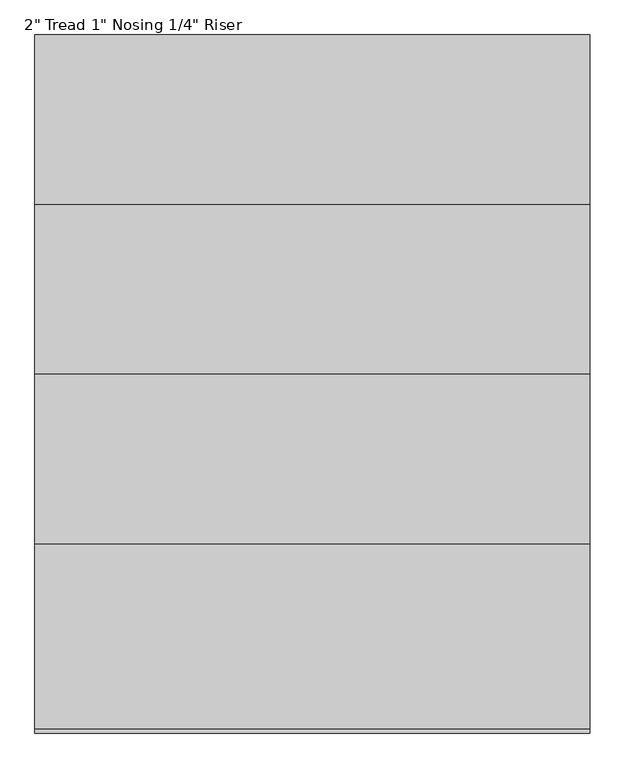
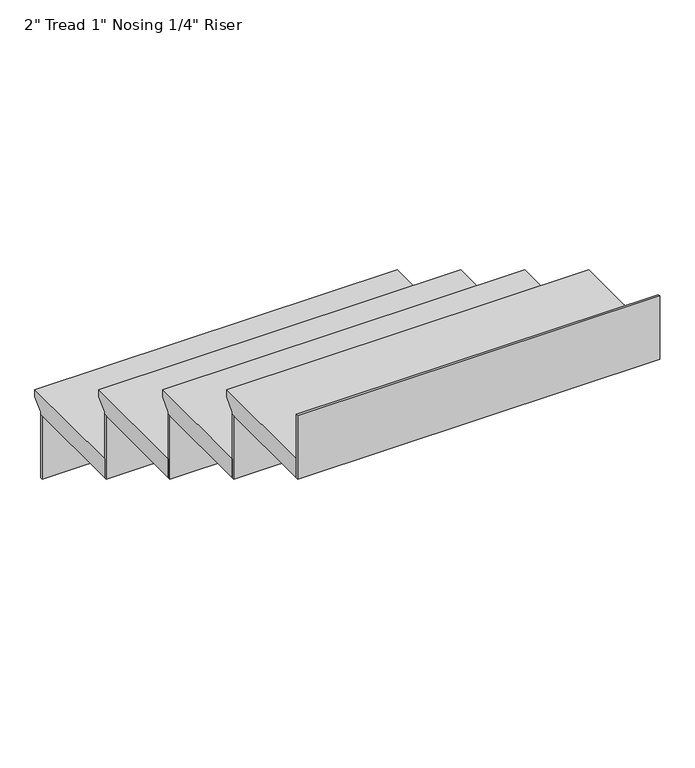
"""IFC4 building model written with IfcOpenShell, lengths in millimetres: stair flight geometry."""

from ifc_helpers import new_model, si_unit, frame, origin, place, context, project, spatial, polyline, outline, extrude, source, transform, mapped, element, save


def stair_flight_d5778488(model_context):
    return source(origin(), model_context, "Body", "SweptSolid", [
        extrude(outline(polyline([(22889.9216096, 45893.2839133), (23194.7216096, 45893.2839133), (23194.7216096, 45874.2339133), (23169.3216096, 45848.8339133), (23169.3216096, 45842.4839133), (22889.9216096, 45842.4839133), (22889.9216096, 45893.2839133)])), frame((-2398.2415084, 0.0, 0.0), z_axis=(1.0, 0.0, 0.0), x_axis=(0.0, 1.0, 0.0)), (0.0, 0.0, 1.0), 914.4),
        extrude(outline(polyline([(-2398.2415084, 23162.9716096), (-2398.2415084, 23169.3216096), (-1483.8415084, 23169.3216096), (-1483.8415084, 23162.9716096), (-2398.2415084, 23162.9716096)])), frame((0.0, 0.0, 45673.1505799), z_axis=(0.0, 0.0, 1.0), x_axis=(1.0, 0.0, 0.0)), (0.0, 0.0, 1.0), 169.3333333),
        extrude(outline(polyline([(-2398.2415084, 22883.5716096), (-2398.2415084, 22889.9216096), (-1483.8415084, 22889.9216096), (-1483.8415084, 22883.5716096), (-2398.2415084, 22883.5716096)])), frame((0.0, 0.0, 45842.4839133), z_axis=(0.0, 0.0, 1.0), x_axis=(1.0, 0.0, 0.0)), (0.0, 0.0, 1.0), 169.3333333),
        extrude(outline(polyline([(22610.5216096, 46062.6172466), (22915.3216096, 46062.6172466), (22915.3216096, 46043.5672466), (22889.9216096, 46018.1672466), (22889.9216096, 46011.8172466), (22610.5216096, 46011.8172466), (22610.5216096, 46062.6172466)])), frame((-2398.2415084, 0.0, 0.0), z_axis=(1.0, 0.0, 0.0), x_axis=(0.0, 1.0, 0.0)), (0.0, 0.0, 1.0), 914.4),
        extrude(outline(polyline([(-2398.2415084, 22604.1716096), (-2398.2415084, 22610.5216096), (-1483.8415084, 22610.5216096), (-1483.8415084, 22604.1716096), (-2398.2415084, 22604.1716096)])), frame((0.0, 0.0, 46011.8172466), z_axis=(0.0, 0.0, 1.0), x_axis=(1.0, 0.0, 0.0)), (0.0, 0.0, 1.0), 169.3333333),
        extrude(outline(polyline([(22331.1216096, 46231.9505799), (22635.9216096, 46231.9505799), (22635.9216096, 46212.9005799), (22610.5216096, 46187.5005799), (22610.5216096, 46181.1505799), (22331.1216096, 46181.1505799), (22331.1216096, 46231.9505799)])), frame((-2398.2415084, 0.0, 0.0), z_axis=(1.0, 0.0, 0.0), x_axis=(0.0, 1.0, 0.0)), (0.0, 0.0, 1.0), 914.4),
        extrude(outline(polyline([(-2398.2415084, 22324.7716096), (-2398.2415084, 22331.1216096), (-1483.8415084, 22331.1216096), (-1483.8415084, 22324.7716096), (-2398.2415084, 22324.7716096)])), frame((0.0, 0.0, 46181.1505799), z_axis=(0.0, 0.0, 1.0), x_axis=(1.0, 0.0, 0.0)), (0.0, 0.0, 1.0), 169.3333333),
        extrude(outline(polyline([(-2398.2415084, 22045.3716096), (-2398.2415084, 22051.7216096), (-1483.8415084, 22051.7216096), (-1483.8415084, 22045.3716096), (-2398.2415084, 22045.3716096)])), frame((0.0, 0.0, 46350.4839133), z_axis=(0.0, 0.0, 1.0), x_axis=(1.0, 0.0, 0.0)), (0.0, 0.0, 1.0), 169.3333333),
        extrude(outline(polyline([(22051.7216096, 46401.2839133), (22356.5216096, 46401.2839133), (22356.5216096, 46382.2339133), (22331.1216096, 46356.8339133), (22331.1216096, 46350.4839133), (22051.7216096, 46350.4839133), (22051.7216096, 46401.2839133)])), frame((-2398.2415084, 0.0, 0.0), z_axis=(1.0, 0.0, 0.0), x_axis=(0.0, 1.0, 0.0)), (0.0, 0.0, 1.0), 914.4),
    ])


if __name__ == "__main__":
    model = new_model("IFC4")
    model_context = context("Model", 3, world=origin())
    ifc_project = project(units=[si_unit("LENGTHUNIT", "METRE", prefix="MILLI")], contexts=[model_context])
    site = spatial("IfcSite", under=ifc_project)
    building = spatial("IfcBuilding", under=site)
    placement = place(None, origin())
    stair_flight_shape = stair_flight_d5778488(model_context)
    element("IfcStairFlight", 1, ObjectType="2\" Tread 1\" Nosing 1/4\" Riser", at=placement, inside=building, context=model_context, shape_type="MappedRepresentation", body=[
        mapped(stair_flight_shape, transform((0.0, 0.0, 0.0), x_axis=(1.0, 0.0, 0.0), y_axis=(0.0, 1.0, 0.0), z_axis=(0.0, 0.0, 1.0))),
    ])
    save(model, "model.ifc")
